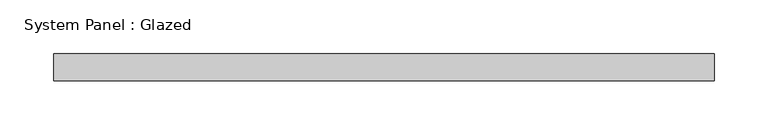
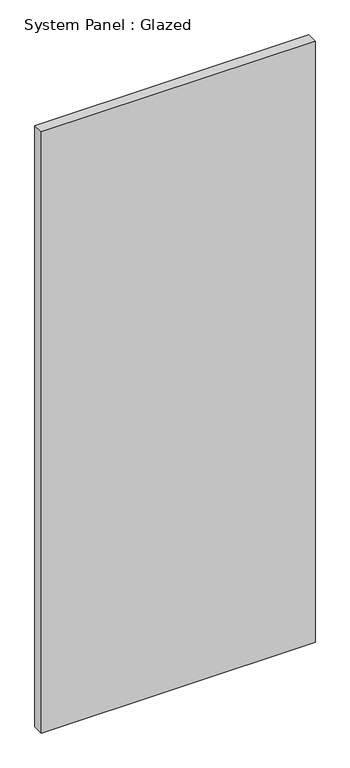
"""IFC4 building model written with IfcOpenShell, lengths in millimetres: plate geometry, System Panel : Glazed."""

from ifc_helpers import new_model, si_unit, origin, origin_with_axes, place, context, project, spatial, polyline, outline, extrude, source, transform, mapped, element, save


def system_panel_glazed_742ba722(model_context):
    return source(origin(), model_context, "Body", "SweptSolid", [
        extrude(outline(polyline([(307.975, 19.05), (-307.975, 19.05), (-307.975, 44.45), (307.975, 44.45), (307.975, 19.05)])), origin_with_axes(), (0.0, 0.0, 1.0), 1430.4533749),
    ])


if __name__ == "__main__":
    model = new_model("IFC4")
    model_context = context("Model", 3, world=origin())
    ifc_project = project(units=[si_unit("LENGTHUNIT", "METRE", prefix="MILLI")], contexts=[model_context])
    site = spatial("IfcSite", under=ifc_project)
    building = spatial("IfcBuilding", under=site)
    placement = place(None, origin())
    system_panel_glazed_shape = system_panel_glazed_742ba722(model_context)
    element("IfcPlate", 1, ObjectType="System Panel : Glazed", at=placement, inside=building, context=model_context, shape_type="MappedRepresentation", body=[
        mapped(system_panel_glazed_shape, transform((0.0, 0.0, 0.0), x_axis=(1.0, 0.0, 0.0), y_axis=(0.0, 1.0, 0.0), z_axis=(0.0, 0.0, 1.0))),
    ])
    save(model, "model.ifc")

# Revit data of these elements
# Type "System Panel : Glazed"
#   Construction Type Id = "GSP4R"
#   Analytic Construction = "1/8 in Pilkington single glazing"
#   Visual Light Transmittance = 0.9
#   Solar Heat Gain Coefficient = 0.86
#   Heat Transfer Coefficient (U) = 1.18115 BTU/(h·ft²·°F)
#   Define Thermal Properties by = 1
# Element 1 (IfcPlate, "System Panel : Glazed")
#   Materials on its faces: "Glass"
# Materials
#   "Glass": class "Glass", colour RGB 0 128 192, transparency 0.75, Description = "Soda Lime Glass", Cost = 0
